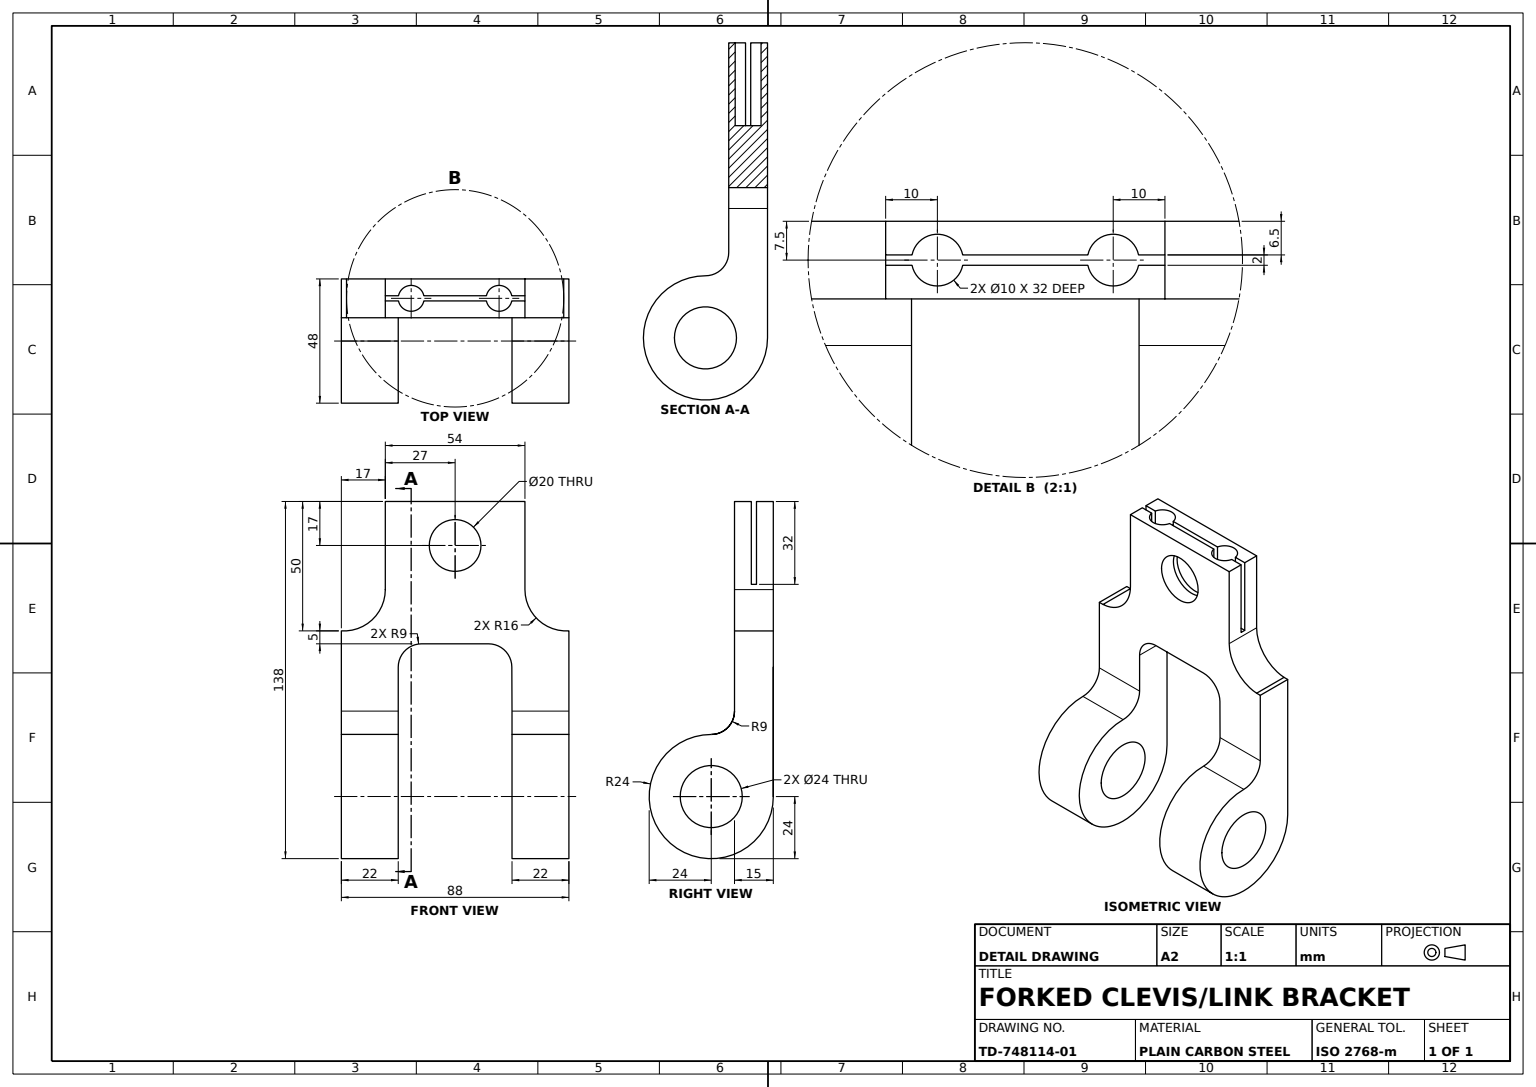
from build123d import *

# Parameters (mm, degrees)
FORK_EYE_PROFILE_R         = 12
FORK_LEG_LEFT_DEPTH        = 22
FORK_START                 = 88
SKETCH1_4_R                = 12
FORK_LEG_RIGHT_DEPTH       = 22
CLAMP_BLOCK_DEPTH          = 15
CROSS_HOLE_SKETCH_R        = 10
CROSS_HOLE_DEPTH           = 15
CLAMP_SLIT_SKETCH_W        = 2
CLAMP_SLIT_SKETCH_H        = 32
CLAMP_SLIT_DEPTH           = 137.429468957
CLAMP_SCREW_HOLES_SKETCH_R = 5
CLAMP_SCREW_HOLES_DEPTH    = 32


with BuildPart() as part:
    # Fork Eye Profile → Fork Leg Left (new body)
    with BuildSketch(Plane(origin=(0, 0, 0), x_dir=(0, 0, -1), z_dir=(1, 0, 0))):
        with BuildLine():
            Line((24, 0), (24, 64))
            Line((24, 64), (9, 64))
            Line((9, 64), (9, 33))
            ThreePointArc((9, 33), (6.363961031, 26.636038969), (0, 24))
            ThreePointArc((0, 24), (-16.970562748, -16.970562748), (24, 0))
        make_face()
        Circle(FORK_EYE_PROFILE_R, mode=Mode.SUBTRACT)
    extrude(amount=FORK_LEG_LEFT_DEPTH)



with BuildPart() as body_2:
    # Sketch1_4 → Fork Leg Right (new body)
    with BuildSketch(Plane(origin=(0, 0, 0), x_dir=(0, 0, -1), z_dir=(1, 0, 0)).offset(FORK_START)):
        with BuildLine():
            Line((24, 0), (24, 64))
            Line((24, 64), (9, 64))
            Line((9, 64), (9, 33))
            ThreePointArc((9, 33), (6.363961031, 26.636038969), (0, 24))
            ThreePointArc((0, 24), (-16.970562748, -16.970562748), (24, 0))
        make_face()
        Circle(SKETCH1_4_R, mode=Mode.SUBTRACT)
    extrude(amount=-FORK_LEG_RIGHT_DEPTH)


with BuildPart() as part_1:
    add(part.part)

    add(body_2.part)  # Clamp Block merges body 2
    # Clamp Block Profile → Clamp Block (add)
    with BuildSketch(Plane.XY.offset(-9)):
        with BuildLine():
            Line((71, 114), (17, 114))
            Line((17, 114), (17, 80))
            ThreePointArc((17, 80), (12.672648111, 69.025683194), (2.000061163, 64))
            Line((2.000061163, 64), (22, 64))
            Line((22, 64), (22, 50))
            ThreePointArc((22, 50), (24.636038969, 56.363961031), (31, 59))
            Line((31, 59), (56.929939565, 59))
            ThreePointArc((56.929939565, 59), (63.280787887, 56.377046776), (65.929863303, 50.03705013))
            Line((65.929863303, 50.03705013), (66, 33))
            Line((66, 33), (88, 33))
            Line((88, 33), (88, 64))
            ThreePointArc((88, 64), (87, 63.968719423), (86, 64))
            ThreePointArc((86, 64), (75.33809621, 69.014268273), (71, 79.968719423))
            Line((71, 79.968719423), (71, 114))
        make_face()
        with BuildLine():
            Line((22, 64), (2.000061163, 64))
            ThreePointArc((2.000061163, 64), (1.000030581, 63.968717508), (0, 64))
            Line((0, 64), (0, 59))
            Line((0, 59), (0, 33))
            Line((0, 33), (22, 33))
            Line((22, 33), (22, 50))
            Line((22, 50), (22, 64))
        make_face()
    extrude(amount=-CLAMP_BLOCK_DEPTH)

    # Cross Hole Sketch → Cross Hole (cut)
    with BuildSketch(Plane.XY.offset(-9)):
        with Locations((44, 97)):
            Circle(CROSS_HOLE_SKETCH_R)
    extrude(amount=-CROSS_HOLE_DEPTH, mode=Mode.SUBTRACT)

    # Clamp Slit Sketch → Clamp Slit (cut, through all)
    with BuildSketch(Plane.ZY.offset(-17)):
        with Locations((-16.5, 98)):
            Rectangle(CLAMP_SLIT_SKETCH_W, CLAMP_SLIT_SKETCH_H)
    extrude(amount=-CLAMP_SLIT_DEPTH, mode=Mode.SUBTRACT)

    # Clamp Screw Holes Sketch → Clamp Screw Holes (cut)
    with BuildSketch(Plane(origin=(0, 114, 0), x_dir=(1, 0, 0), z_dir=(0, 1, 0))):
        with Locations((27, 16.5)):
            Circle(CLAMP_SCREW_HOLES_SKETCH_R)
        with Locations((61, 16.5)):
            Circle(CLAMP_SCREW_HOLES_SKETCH_R)
    extrude(amount=-CLAMP_SCREW_HOLES_DEPTH, mode=Mode.SUBTRACT)


solid = part_1.part
